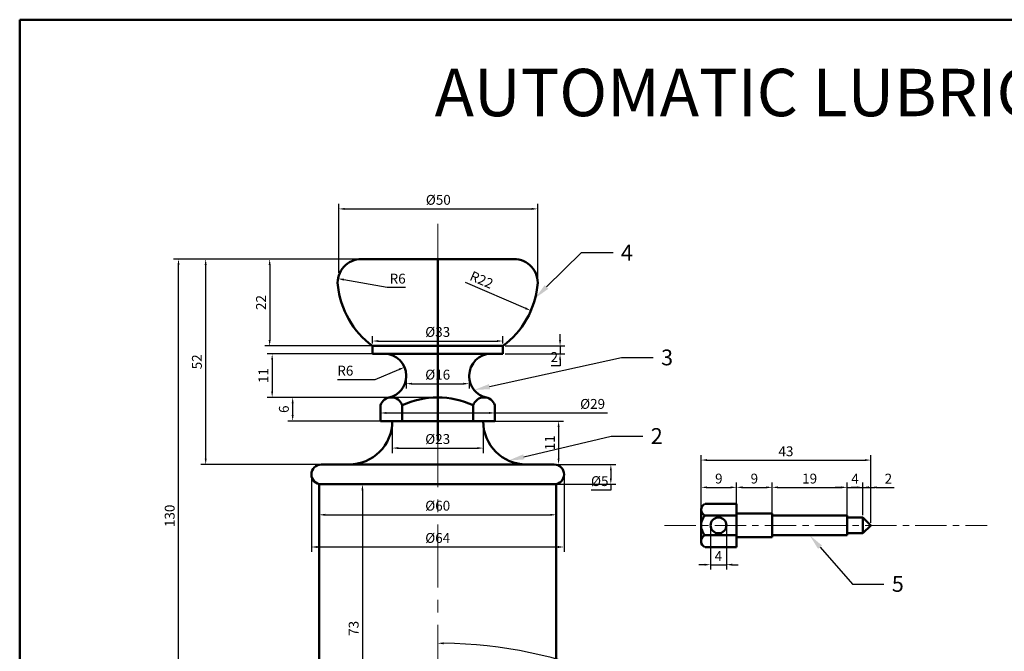
# Model space of a CAD drawing. Units: millimetres. Extents: x -414 to 17, y 81 to 417.
# Tile 6 of 7: x -414 to -165, y 257 to 417. Entities that reach past the tile are written whole.
import ezdxf
from ezdxf import colors
from ezdxf.entities.mleader import LeaderData, LeaderLine
from ezdxf.math import Vec2, Vec3

# ---------------------------------------------------------------- set-up
doc = ezdxf.new("R2010")
doc.units = ezdxf.units.MM
doc.header["$LTSCALE"] = 0.5
doc.linetypes.add('CENTER', pattern=[50.8, 31.75, -6.35, 6.35, -6.35])
for name, color, linetype, lineweight in [('M-CNTR', 1, 'CENTER', 18), ('M-DIMS', 2, 'Continuous', 25), ('M-OUTL', 7, 'Continuous', 50), ('M-TEXT', 3, 'Continuous', 25)]:
    doc.layers.add(name, color=color, linetype=linetype, lineweight=lineweight)
doc.styles.get("Standard").update_dxf_attribs({"font": 'arial.ttf'})
doc.dimstyles.new('ISO-25', dxfattribs={"dimtxt": 2.5, "dimasz": 1.5, "dimexe": 1.25, "dimexo": 0.625, "dimtad": 1, "dimtoh": 1, "dimdec": 0, "dimtxsty": 'Standard', "dimcen": 2.5, "dimadec": 0, "dimazin": 0, "dimtfac": 1, "dimtdec": 0, "dimtmove": 0, "dimatfit": 3, "dimfxl": 1, "dimarcsym": 0})

# ---------------------------------------------------------------- blocks, each defined once
blk = doc.blocks.new('*D1')
at = {"layer": 'Defpoints', "color": 0, "ltscale": 0.5, "transparency": 16777216}
for p in [(-283.16, 369.18), (-333.52, 352.37), (-283.16, 350.47)]:
    blk.add_point(p, dxfattribs=at)
at = {"layer": 'M-DIMS', "color": 0, "lineweight": -2, "ltscale": 0.5, "transparency": 16777216}
for p, q in [((-333.52, 353), (-333.52, 370.43)), ((-332.02, 369.18), (-284.66, 369.18)), ((-283.16, 351.09), (-283.16, 370.43))]:
    blk.add_line(p, q, dxfattribs=at)
at = {"layer": 'M-DIMS', "color": 0, "ltscale": 0.5, "transparency": 16777216}
for points in [[(-332.02, 369.43), (-332.02, 368.93), (-333.52, 369.18)], [(-284.66, 369.43), (-284.66, 368.93), (-283.16, 369.18)]]:
    blk.add_solid(points, dxfattribs=at)
at = {"layer": 'M-DIMS', "color": 0, "ltscale": 0.5, "transparency": 16777216, "insert": (-308.34, 371.15), "char_height": 2.5, "attachment_point": 5}
blk.add_mtext('%%C50', dxfattribs=at)
blk = doc.blocks.new('*D2')
at = {"layer": 'Defpoints', "color": 0, "ltscale": 0.5, "transparency": 16777216}
for p in [(-367.26, 356.47), (-319.11, 356.47), (-319.11, 304.46)]:
    blk.add_point(p, dxfattribs=at)
at = {"layer": 'M-DIMS', "color": 0, "lineweight": -2, "ltscale": 0.5, "transparency": 16777216}
for p, q in [((-319.74, 356.47), (-368.51, 356.47)), ((-367.26, 305.96), (-367.26, 354.97)), ((-319.74, 304.46), (-368.51, 304.46))]:
    blk.add_line(p, q, dxfattribs=at)
at = {"layer": 'M-DIMS', "color": 0, "ltscale": 0.5, "transparency": 16777216}
for points in [[(-367.51, 354.97), (-367.01, 354.97), (-367.26, 356.47)], [(-367.51, 305.96), (-367.01, 305.96), (-367.26, 304.46)]]:
    blk.add_solid(points, dxfattribs=at)
at = {"layer": 'M-DIMS', "color": 0, "ltscale": 0.5, "transparency": 16777216, "insert": (-369.16, 330.46), "char_height": 2.5, "attachment_point": 5, "rotation": 90}
blk.add_mtext('52', dxfattribs=at)
blk = doc.blocks.new('*D3')
at = {"layer": 'Defpoints', "color": 0, "ltscale": 0.5, "transparency": 16777216}
for p in [(-339.99, 356.47), (-351.05, 334.47), (-315.35, 334.47)]:
    blk.add_point(p, dxfattribs=at)
at = {"layer": 'M-DIMS', "color": 0, "lineweight": -2, "ltscale": 0.5, "transparency": 16777216}
for p, q in [((-340.61, 356.47), (-352.3, 356.47)), ((-351.05, 354.97), (-351.05, 335.97)), ((-315.97, 334.47), (-352.3, 334.47))]:
    blk.add_line(p, q, dxfattribs=at)
at = {"layer": 'M-DIMS', "color": 0, "ltscale": 0.5, "transparency": 16777216}
for points in [[(-351.3, 354.97), (-350.8, 354.97), (-351.05, 356.47)], [(-351.3, 335.97), (-350.8, 335.97), (-351.05, 334.47)]]:
    blk.add_solid(points, dxfattribs=at)
at = {"layer": 'M-DIMS', "color": 0, "ltscale": 0.5, "transparency": 16777216, "insert": (-352.93, 345.47), "char_height": 2.5, "attachment_point": 5, "rotation": 90}
blk.add_mtext('22', dxfattribs=at)
blk = doc.blocks.new('*D4')
at = {"layer": 'Defpoints', "color": 0, "ltscale": 0.5, "transparency": 16777216}
for p in [(-291.99, 334.47), (-291.99, 332.47), (-277.5, 332.47)]:
    blk.add_point(p, dxfattribs=at)
at = {"layer": 'M-DIMS', "color": 0, "lineweight": -2, "ltscale": 0.5, "transparency": 16777216}
for p, q in [((-277.5, 335.97), (-277.5, 337.47)), ((-291.37, 334.47), (-276.25, 334.47)), ((-277.5, 334.47), (-277.5, 332.47)), ((-291.37, 332.47), (-276.25, 332.47)), ((-277.5, 329.47), (-279.78, 329.47)), ((-277.5, 330.97), (-277.5, 329.47))]:
    blk.add_line(p, q, dxfattribs=at)
at = {"layer": 'M-DIMS', "color": 0, "ltscale": 0.5, "transparency": 16777216}
for points in [[(-277.75, 335.97), (-277.25, 335.97), (-277.5, 334.47)], [(-277.75, 330.97), (-277.25, 330.97), (-277.5, 332.47)]]:
    blk.add_solid(points, dxfattribs=at)
at = {"layer": 'M-DIMS', "color": 0, "ltscale": 0.5, "transparency": 16777216, "insert": (-278.95, 331.35), "char_height": 2.5, "attachment_point": 5}
blk.add_mtext('2', dxfattribs=at)
blk = doc.blocks.new('*D5')
at = {"layer": 'Defpoints', "color": 0, "ltscale": 0.5, "transparency": 16777216}
for p in [(-316.49, 326.78), (-300.49, 326.78), (-300.49, 324.92)]:
    blk.add_point(p, dxfattribs=at)
at = {"layer": 'M-DIMS', "color": 0, "lineweight": -2, "ltscale": 0.5, "transparency": 16777216}
for p, q in [((-316.49, 326.15), (-316.49, 323.67)), ((-314.99, 324.92), (-301.99, 324.92)), ((-300.49, 326.15), (-300.49, 323.67))]:
    blk.add_line(p, q, dxfattribs=at)
at = {"layer": 'M-DIMS', "color": 0, "ltscale": 0.5, "transparency": 16777216}
for points in [[(-314.99, 325.17), (-314.99, 324.67), (-316.49, 324.92)], [(-301.99, 325.17), (-301.99, 324.67), (-300.49, 324.92)]]:
    blk.add_solid(points, dxfattribs=at)
at = {"layer": 'M-DIMS', "color": 0, "ltscale": 0.5, "transparency": 16777216, "insert": (-308.49, 326.89), "char_height": 2.5, "attachment_point": 5}
blk.add_mtext('%%C16', dxfattribs=at)
blk = doc.blocks.new('*D6')
at = {"layer": 'Defpoints', "color": 0, "ltscale": 0.5, "transparency": 16777216}
for p in [(-308.49, 332.47), (-350.42, 321.46), (-308.49, 321.46)]:
    blk.add_point(p, dxfattribs=at)
at = {"layer": 'M-DIMS', "color": 0, "lineweight": -2, "ltscale": 0.5, "transparency": 16777216}
for p, q in [((-309.12, 332.47), (-351.67, 332.47)), ((-350.42, 330.97), (-350.42, 322.96)), ((-309.12, 321.46), (-351.67, 321.46))]:
    blk.add_line(p, q, dxfattribs=at)
at = {"layer": 'M-DIMS', "color": 0, "ltscale": 0.5, "transparency": 16777216}
for points in [[(-350.67, 330.97), (-350.17, 330.97), (-350.42, 332.47)], [(-350.67, 322.96), (-350.17, 322.96), (-350.42, 321.46)]]:
    blk.add_solid(points, dxfattribs=at)
at = {"layer": 'M-DIMS', "color": 0, "ltscale": 0.5, "transparency": 16777216, "insert": (-352.31, 326.96), "char_height": 2.5, "attachment_point": 5, "rotation": 90}
blk.add_mtext('11', dxfattribs=at)
blk = doc.blocks.new('*D7')
at = {"layer": 'Defpoints', "color": 0, "ltscale": 0.5, "transparency": 16777216}
for p in [(-308.49, 321.46), (-345.23, 315.46), (-308.49, 315.46)]:
    blk.add_point(p, dxfattribs=at)
at = {"layer": 'M-DIMS', "color": 0, "lineweight": -2, "ltscale": 0.5, "transparency": 16777216}
for p, q in [((-309.12, 321.46), (-346.48, 321.46)), ((-345.23, 319.96), (-345.23, 316.96)), ((-309.12, 315.46), (-346.48, 315.46))]:
    blk.add_line(p, q, dxfattribs=at)
at = {"layer": 'M-DIMS', "color": 0, "ltscale": 0.5, "transparency": 16777216}
for points in [[(-345.48, 319.96), (-344.98, 319.96), (-345.23, 321.46)], [(-345.48, 316.96), (-344.98, 316.96), (-345.23, 315.46)]]:
    blk.add_solid(points, dxfattribs=at)
at = {"layer": 'M-DIMS', "color": 0, "ltscale": 0.5, "transparency": 16777216, "insert": (-347.13, 318.46), "char_height": 2.5, "attachment_point": 5, "rotation": 90}
blk.add_mtext('6', dxfattribs=at)
blk = doc.blocks.new('*D8')
at = {"layer": 'Defpoints', "color": 0, "ltscale": 0.5, "transparency": 16777216}
for p in [(-308.49, 315.46), (-308.49, 304.46), (-277.87, 304.46)]:
    blk.add_point(p, dxfattribs=at)
at = {"layer": 'M-DIMS', "color": 0, "lineweight": -2, "ltscale": 0.5, "transparency": 16777216}
for p, q in [((-307.87, 315.46), (-276.62, 315.46)), ((-277.87, 313.96), (-277.87, 305.96)), ((-307.87, 304.46), (-276.62, 304.46))]:
    blk.add_line(p, q, dxfattribs=at)
at = {"layer": 'M-DIMS', "color": 0, "ltscale": 0.5, "transparency": 16777216}
for points in [[(-278.12, 313.96), (-277.62, 313.96), (-277.87, 315.46)], [(-278.12, 305.96), (-277.62, 305.96), (-277.87, 304.46)]]:
    blk.add_solid(points, dxfattribs=at)
at = {"layer": 'M-DIMS', "color": 0, "ltscale": 0.5, "transparency": 16777216, "insert": (-279.75, 309.96), "char_height": 2.5, "attachment_point": 5, "rotation": 90}
blk.add_mtext('11', dxfattribs=at)
blk = doc.blocks.new('*D9')
at = {"layer": 'Defpoints', "color": 0, "ltscale": 0.5, "transparency": 16777216}
for p in [(-324.99, 334.47), (-291.99, 335.72), (-291.99, 334.47)]:
    blk.add_point(p, dxfattribs=at)
at = {"layer": 'M-DIMS', "color": 0, "lineweight": -2, "ltscale": 0.5, "transparency": 16777216}
for p, q in [((-324.99, 335.09), (-324.99, 336.97)), ((-291.99, 335.09), (-291.99, 336.97)), ((-323.49, 335.72), (-293.49, 335.72))]:
    blk.add_line(p, q, dxfattribs=at)
at = {"layer": 'M-DIMS', "color": 0, "ltscale": 0.5, "transparency": 16777216}
for points in [[(-323.49, 335.97), (-323.49, 335.47), (-324.99, 335.72)], [(-293.49, 335.97), (-293.49, 335.47), (-291.99, 335.72)]]:
    blk.add_solid(points, dxfattribs=at)
at = {"layer": 'M-DIMS', "color": 0, "ltscale": 0.5, "transparency": 16777216, "insert": (-308.49, 337.7), "char_height": 2.5, "attachment_point": 5}
blk.add_mtext('%%C33', dxfattribs=at)
blk = doc.blocks.new('*D10')
at = {"layer": 'Defpoints', "color": 0, "ltscale": 0.5, "transparency": 16777216}
for p in [(-333.74, 351.52), (-327.83, 350.47)]:
    blk.add_point(p, dxfattribs=at)
at = {"layer": 'M-DIMS', "color": 0, "lineweight": -2, "ltscale": 0.5, "transparency": 16777216}
for p, q in [((-321.28, 349.3), (-332.26, 351.26)), ((-316.62, 349.3), (-321.28, 349.3))]:
    blk.add_line(p, q, dxfattribs=at)
at = {"layer": 'M-DIMS', "color": 0, "ltscale": 0.5, "transparency": 16777216}
blk.add_solid([(-332.22, 351.5), (-332.3, 351.01), (-333.74, 351.52)], dxfattribs=at)
at = {"layer": 'M-DIMS', "color": 0, "ltscale": 0.5, "transparency": 16777216, "insert": (-318.64, 351.2), "char_height": 2.5, "attachment_point": 5}
blk.add_mtext('R6', dxfattribs=at)
blk = doc.blocks.new('*D11')
at = {"layer": 'Defpoints', "color": 0, "ltscale": 0.5, "transparency": 16777216}
for p in [(-305.07, 352.16), (-284.88, 343.42)]:
    blk.add_point(p, dxfattribs=at)
at = {"layer": 'M-DIMS', "color": 0, "lineweight": -2, "ltscale": 0.5, "transparency": 16777216}
blk.add_line((-301.55, 350.64), (-286.26, 344.01), dxfattribs=at)
at = {"layer": 'M-DIMS', "color": 0, "ltscale": 0.5, "transparency": 16777216}
blk.add_solid([(-286.16, 344.24), (-286.36, 343.78), (-284.88, 343.42)], dxfattribs=at)
at = {"layer": 'M-DIMS', "color": 0, "ltscale": 0.5, "transparency": 16777216, "insert": (-297.5, 350.93), "char_height": 2.5, "attachment_point": 5, "rotation": 336.5806}
blk.add_mtext('R22', dxfattribs=at)
blk = doc.blocks.new('*D12')
at = {"layer": 'Defpoints', "color": 0, "ltscale": 0.5, "transparency": 16777216}
for p in [(-321.99, 326.97), (-316.92, 329.09)]:
    blk.add_point(p, dxfattribs=at)
at = {"layer": 'M-DIMS', "color": 0, "lineweight": -2, "ltscale": 0.5, "transparency": 16777216}
for p, q in [((-324.3, 326), (-318.3, 328.51)), ((-333.9, 326), (-324.3, 326))]:
    blk.add_line(p, q, dxfattribs=at)
at = {"layer": 'M-DIMS', "color": 0, "ltscale": 0.5, "transparency": 16777216}
blk.add_solid([(-318.4, 328.74), (-318.21, 328.28), (-316.92, 329.09)], dxfattribs=at)
at = {"layer": 'M-DIMS', "color": 0, "ltscale": 0.5, "transparency": 16777216, "insert": (-331.89, 327.9), "char_height": 2.5, "attachment_point": 5}
blk.add_mtext('R6', dxfattribs=at)
blk = doc.blocks.new('*D13')
at = {"layer": 'Defpoints', "color": 0, "ltscale": 0.5, "transparency": 16777216}
for p in [(-293.99, 317.51), (-322.99, 315.46), (-293.99, 315.46)]:
    blk.add_point(p, dxfattribs=at)
at = {"layer": 'M-DIMS', "color": 0, "lineweight": -2, "ltscale": 0.5, "transparency": 16777216}
for p, q in [((-322.99, 316.09), (-322.99, 318.76)), ((-321.49, 317.51), (-295.49, 317.51)), ((-293.99, 316.09), (-293.99, 318.76)), ((-293.99, 317.51), (-265.48, 317.51))]:
    blk.add_line(p, q, dxfattribs=at)
at = {"layer": 'M-DIMS', "color": 0, "ltscale": 0.5, "transparency": 16777216}
for points in [[(-321.49, 317.76), (-321.49, 317.26), (-322.99, 317.51)], [(-295.49, 317.76), (-295.49, 317.26), (-293.99, 317.51)]]:
    blk.add_solid(points, dxfattribs=at)
at = {"layer": 'M-DIMS', "color": 0, "ltscale": 0.5, "transparency": 16777216, "insert": (-269.26, 319.48), "char_height": 2.5, "attachment_point": 5}
blk.add_mtext('%%C29', dxfattribs=at)
blk = doc.blocks.new('*D14')
at = {"layer": 'Defpoints', "color": 0, "ltscale": 0.5, "transparency": 16777216}
for p in [(-319.99, 315.46), (-296.99, 315.46), (-296.99, 308.62)]:
    blk.add_point(p, dxfattribs=at)
at = {"layer": 'M-DIMS', "color": 0, "lineweight": -2, "ltscale": 0.5, "transparency": 16777216}
for p, q in [((-319.99, 314.84), (-319.99, 307.37)), ((-296.99, 314.84), (-296.99, 307.37)), ((-318.49, 308.62), (-298.49, 308.62))]:
    blk.add_line(p, q, dxfattribs=at)
at = {"layer": 'M-DIMS', "color": 0, "ltscale": 0.5, "transparency": 16777216}
for points in [[(-318.49, 308.87), (-318.49, 308.37), (-319.99, 308.62)], [(-298.49, 308.87), (-298.49, 308.37), (-296.99, 308.62)]]:
    blk.add_solid(points, dxfattribs=at)
at = {"layer": 'M-DIMS', "color": 0, "ltscale": 0.5, "transparency": 16777216, "insert": (-308.49, 310.59), "char_height": 2.5, "attachment_point": 5}
blk.add_mtext('%%C23', dxfattribs=at)
blk = doc.blocks.new('*D15')
at = {"layer": 'Defpoints', "color": 0, "ltscale": 0.5, "transparency": 16777216}
for p in [(-282.49, 304.46), (-282.49, 299.46), (-264.64, 299.46)]:
    blk.add_point(p, dxfattribs=at)
at = {"layer": 'M-DIMS', "color": 0, "lineweight": -2, "ltscale": 0.5, "transparency": 16777216}
for p, q in [((-281.87, 304.46), (-263.39, 304.46)), ((-264.64, 302.96), (-264.64, 300.96)), ((-281.87, 299.46), (-263.39, 299.46)), ((-264.64, 299.46), (-264.64, 297.96)), ((-264.64, 297.96), (-269.64, 297.96))]:
    blk.add_line(p, q, dxfattribs=at)
at = {"layer": 'M-DIMS', "color": 0, "ltscale": 0.5, "transparency": 16777216}
for points in [[(-264.89, 302.96), (-264.39, 302.96), (-264.64, 304.46)], [(-264.89, 300.96), (-264.39, 300.96), (-264.64, 299.46)]]:
    blk.add_solid(points, dxfattribs=at)
at = {"layer": 'M-DIMS', "color": 0, "ltscale": 0.5, "transparency": 16777216, "insert": (-267.45, 299.93), "char_height": 2.5, "attachment_point": 5}
blk.add_mtext('%%C5', dxfattribs=at)
blk = doc.blocks.new('*D16')
at = {"layer": 'Defpoints', "color": 0, "ltscale": 0.5, "transparency": 16777216}
for p in [(-340.49, 301.96), (-276.49, 301.96), (-276.49, 283.57)]:
    blk.add_point(p, dxfattribs=at)
at = {"layer": 'M-DIMS', "color": 0, "lineweight": -2, "ltscale": 0.5, "transparency": 16777216}
for p, q in [((-340.49, 301.34), (-340.49, 282.32)), ((-276.49, 301.34), (-276.49, 282.32)), ((-338.99, 283.57), (-277.99, 283.57))]:
    blk.add_line(p, q, dxfattribs=at)
at = {"layer": 'M-DIMS', "color": 0, "ltscale": 0.5, "transparency": 16777216}
for points in [[(-338.99, 283.82), (-338.99, 283.32), (-340.49, 283.57)], [(-277.99, 283.82), (-277.99, 283.32), (-276.49, 283.57)]]:
    blk.add_solid(points, dxfattribs=at)
at = {"layer": 'M-DIMS', "color": 0, "ltscale": 0.5, "transparency": 16777216, "insert": (-308.49, 285.54), "char_height": 2.5, "attachment_point": 5}
blk.add_mtext('%%C64', dxfattribs=at)
blk = doc.blocks.new('*D17')
at = {"layer": 'Defpoints', "color": 0, "ltscale": 0.5, "transparency": 16777216}
for p in [(-338.49, 294.85), (-278.49, 294.85), (-278.49, 291.72)]:
    blk.add_point(p, dxfattribs=at)
at = {"layer": 'M-DIMS', "color": 0, "lineweight": -2, "ltscale": 0.5, "transparency": 16777216}
for p, q in [((-338.49, 294.23), (-338.49, 290.47)), ((-278.49, 294.23), (-278.49, 290.47)), ((-336.99, 291.72), (-279.99, 291.72))]:
    blk.add_line(p, q, dxfattribs=at)
at = {"layer": 'M-DIMS', "color": 0, "ltscale": 0.5, "transparency": 16777216}
for points in [[(-336.99, 291.97), (-336.99, 291.47), (-338.49, 291.72)], [(-279.99, 291.97), (-279.99, 291.47), (-278.49, 291.72)]]:
    blk.add_solid(points, dxfattribs=at)
at = {"layer": 'M-DIMS', "color": 0, "ltscale": 0.5, "transparency": 16777216, "insert": (-308.49, 293.7), "char_height": 2.5, "attachment_point": 5}
blk.add_mtext('%%C60', dxfattribs=at)
blk = doc.blocks.new('*D18')
at = {"layer": 'Defpoints', "color": 0, "ltscale": 0.5, "transparency": 16777216}
for p in [(-328.26, 299.46), (-328.26, 226.46), (-327.55, 226.46)]:
    blk.add_point(p, dxfattribs=at)
at = {"layer": 'M-DIMS', "color": 0, "lineweight": -2, "ltscale": 0.5, "transparency": 16777216}
for p, q in [((-327.63, 299.46), (-326.3, 299.46)), ((-327.55, 297.96), (-327.55, 227.96)), ((-327.63, 226.46), (-326.3, 226.46))]:
    blk.add_line(p, q, dxfattribs=at)
at = {"layer": 'M-DIMS', "color": 0, "ltscale": 0.5, "transparency": 16777216}
for points in [[(-327.8, 297.96), (-327.3, 297.96), (-327.55, 299.46)], [(-327.8, 227.96), (-327.3, 227.96), (-327.55, 226.46)]]:
    blk.add_solid(points, dxfattribs=at)
at = {"layer": 'M-DIMS', "color": 0, "ltscale": 0.5, "transparency": 16777216, "insert": (-329.45, 262.96), "char_height": 2.5, "attachment_point": 5, "rotation": 90}
blk.add_mtext('73', dxfattribs=at)
blk = doc.blocks.new('*D39')
at = {"layer": 'Defpoints', "color": 0, "ltscale": 0.5, "transparency": 16777216}
for p in [(-374.14, 356.47), (-308.49, 356.47), (-361.11, 226.46)]:
    blk.add_point(p, dxfattribs=at)
at = {"layer": 'M-DIMS', "color": 0, "lineweight": -2, "ltscale": 0.5, "transparency": 16777216}
for p, q in [((-309.12, 356.47), (-375.39, 356.47)), ((-374.14, 227.96), (-374.14, 354.97)), ((-361.74, 226.46), (-375.39, 226.46))]:
    blk.add_line(p, q, dxfattribs=at)
at = {"layer": 'M-DIMS', "color": 0, "ltscale": 0.5, "transparency": 16777216}
for points in [[(-374.39, 354.97), (-373.89, 354.97), (-374.14, 356.47)], [(-374.39, 227.96), (-373.89, 227.96), (-374.14, 226.46)]]:
    blk.add_solid(points, dxfattribs=at)
at = {"layer": 'M-DIMS', "color": 0, "ltscale": 0.5, "transparency": 16777216, "insert": (-376.05, 291.46), "char_height": 2.5, "attachment_point": 5, "rotation": 90}
blk.add_mtext('130', dxfattribs=at)
blk = doc.blocks.new('*D71')
at = {"layer": 'Defpoints', "color": 0, "ltscale": 0.5, "transparency": 16777216}
for p in [(-198.79, 305.58), (-241.79, 289.04), (-198.79, 289.04)]:
    blk.add_point(p, dxfattribs=at)
at = {"layer": 'M-DIMS', "color": 0, "lineweight": -2, "ltscale": 0.5, "transparency": 16777216}
for p, q in [((-241.79, 289.67), (-241.79, 306.83)), ((-198.79, 289.67), (-198.79, 306.83)), ((-240.29, 305.58), (-200.29, 305.58))]:
    blk.add_line(p, q, dxfattribs=at)
at = {"layer": 'M-DIMS', "color": 0, "ltscale": 0.5, "transparency": 16777216}
for points in [[(-240.29, 305.83), (-240.29, 305.33), (-241.79, 305.58)], [(-200.29, 305.83), (-200.29, 305.33), (-198.79, 305.58)]]:
    blk.add_solid(points, dxfattribs=at)
at = {"layer": 'M-DIMS', "color": 0, "ltscale": 0.5, "transparency": 16777216, "insert": (-220.29, 307.48), "char_height": 2.5, "attachment_point": 5}
blk.add_mtext('43', dxfattribs=at)
blk = doc.blocks.new('*D72')
at = {"layer": 'Defpoints', "color": 0, "ltscale": 0.5, "transparency": 16777216}
for p in [(-232.79, 298.67), (-241.79, 289.04), (-232.79, 289.04)]:
    blk.add_point(p, dxfattribs=at)
at = {"layer": 'M-DIMS', "color": 0, "lineweight": -2, "ltscale": 0.5, "transparency": 16777216}
for p, q in [((-241.79, 289.67), (-241.79, 299.92)), ((-232.79, 289.67), (-232.79, 299.92)), ((-240.29, 298.67), (-234.29, 298.67))]:
    blk.add_line(p, q, dxfattribs=at)
at = {"layer": 'M-DIMS', "color": 0, "ltscale": 0.5, "transparency": 16777216}
for points in [[(-240.29, 298.92), (-240.29, 298.42), (-241.79, 298.67)], [(-234.29, 298.92), (-234.29, 298.42), (-232.79, 298.67)]]:
    blk.add_solid(points, dxfattribs=at)
at = {"layer": 'M-DIMS', "color": 0, "ltscale": 0.5, "transparency": 16777216, "insert": (-237.29, 300.57), "char_height": 2.5, "attachment_point": 5}
blk.add_mtext('9', dxfattribs=at)
blk = doc.blocks.new('*D73')
at = {"layer": 'Defpoints', "color": 0, "ltscale": 0.5, "transparency": 16777216}
for p in [(-223.79, 298.67), (-232.79, 289.04), (-223.79, 289.04)]:
    blk.add_point(p, dxfattribs=at)
at = {"layer": 'M-DIMS', "color": 0, "lineweight": -2, "ltscale": 0.5, "transparency": 16777216}
for p, q in [((-232.79, 289.67), (-232.79, 299.92)), ((-223.79, 289.67), (-223.79, 299.92)), ((-231.29, 298.67), (-225.29, 298.67))]:
    blk.add_line(p, q, dxfattribs=at)
at = {"layer": 'M-DIMS', "color": 0, "ltscale": 0.5, "transparency": 16777216}
for points in [[(-231.29, 298.92), (-231.29, 298.42), (-232.79, 298.67)], [(-225.29, 298.92), (-225.29, 298.42), (-223.79, 298.67)]]:
    blk.add_solid(points, dxfattribs=at)
at = {"layer": 'M-DIMS', "color": 0, "ltscale": 0.5, "transparency": 16777216, "insert": (-228.29, 300.57), "char_height": 2.5, "attachment_point": 5}
blk.add_mtext('9', dxfattribs=at)
blk = doc.blocks.new('*D74')
at = {"layer": 'Defpoints', "color": 0, "ltscale": 0.5, "transparency": 16777216}
for p in [(-204.79, 298.67), (-223.79, 289.04), (-204.79, 289.04)]:
    blk.add_point(p, dxfattribs=at)
at = {"layer": 'M-DIMS', "color": 0, "lineweight": -2, "ltscale": 0.5, "transparency": 16777216}
for p, q in [((-223.79, 289.67), (-223.79, 299.92)), ((-204.79, 289.67), (-204.79, 299.92)), ((-222.29, 298.67), (-206.29, 298.67))]:
    blk.add_line(p, q, dxfattribs=at)
at = {"layer": 'M-DIMS', "color": 0, "ltscale": 0.5, "transparency": 16777216}
for points in [[(-222.29, 298.92), (-222.29, 298.42), (-223.79, 298.67)], [(-206.29, 298.92), (-206.29, 298.42), (-204.79, 298.67)]]:
    blk.add_solid(points, dxfattribs=at)
at = {"layer": 'M-DIMS', "color": 0, "ltscale": 0.5, "transparency": 16777216, "insert": (-214.29, 300.57), "char_height": 2.5, "attachment_point": 5}
blk.add_mtext('19', dxfattribs=at)
blk = doc.blocks.new('*D75')
at = {"layer": 'Defpoints', "color": 0, "ltscale": 0.5, "transparency": 16777216}
for p in [(-200.79, 298.67), (-204.79, 291.04), (-200.79, 291.04)]:
    blk.add_point(p, dxfattribs=at)
at = {"layer": 'M-DIMS', "color": 0, "lineweight": -2, "ltscale": 0.5, "transparency": 16777216}
for p, q in [((-204.79, 291.67), (-204.79, 299.92)), ((-200.79, 291.67), (-200.79, 299.92)), ((-206.29, 298.67), (-207.79, 298.67)), ((-204.79, 298.67), (-200.79, 298.67)), ((-199.29, 298.67), (-197.79, 298.67))]:
    blk.add_line(p, q, dxfattribs=at)
at = {"layer": 'M-DIMS', "color": 0, "ltscale": 0.5, "transparency": 16777216}
for points in [[(-206.29, 298.92), (-206.29, 298.42), (-204.79, 298.67)], [(-199.29, 298.92), (-199.29, 298.42), (-200.79, 298.67)]]:
    blk.add_solid(points, dxfattribs=at)
at = {"layer": 'M-DIMS', "color": 0, "ltscale": 0.5, "transparency": 16777216, "insert": (-202.79, 300.54), "char_height": 2.5, "attachment_point": 5}
blk.add_mtext('4', dxfattribs=at)
blk = doc.blocks.new('*D76')
at = {"layer": 'Defpoints', "color": 0, "ltscale": 0.5, "transparency": 16777216}
for p in [(-198.79, 298.67), (-200.79, 291.04), (-198.79, 290.27)]:
    blk.add_point(p, dxfattribs=at)
at = {"layer": 'M-DIMS', "color": 0, "lineweight": -2, "ltscale": 0.5, "transparency": 16777216}
for p, q in [((-200.79, 291.67), (-200.79, 299.92)), ((-198.79, 290.9), (-198.79, 299.92)), ((-202.29, 298.67), (-203.79, 298.67)), ((-200.79, 298.67), (-198.79, 298.67)), ((-197.29, 298.67), (-192.89, 298.67))]:
    blk.add_line(p, q, dxfattribs=at)
at = {"layer": 'M-DIMS', "color": 0, "ltscale": 0.5, "transparency": 16777216}
for points in [[(-202.29, 298.92), (-202.29, 298.42), (-200.79, 298.67)], [(-197.29, 298.92), (-197.29, 298.42), (-198.79, 298.67)]]:
    blk.add_solid(points, dxfattribs=at)
at = {"layer": 'M-DIMS', "color": 0, "ltscale": 0.5, "transparency": 16777216, "insert": (-194.34, 300.55), "char_height": 2.5, "attachment_point": 5}
blk.add_mtext('2', dxfattribs=at)
blk = doc.blocks.new('*D77')
at = {"layer": 'Defpoints', "color": 0, "ltscale": 0.5, "transparency": 16777216}
for p in [(-239.38, 289.04), (-235.38, 289.04), (-235.38, 279.09)]:
    blk.add_point(p, dxfattribs=at)
at = {"layer": 'M-DIMS', "color": 0, "lineweight": -2, "ltscale": 0.5, "transparency": 16777216}
for p, q in [((-239.38, 288.42), (-239.38, 277.84)), ((-235.38, 288.42), (-235.38, 277.84)), ((-240.88, 279.09), (-242.38, 279.09)), ((-239.38, 279.09), (-235.38, 279.09)), ((-233.88, 279.09), (-232.38, 279.09))]:
    blk.add_line(p, q, dxfattribs=at)
at = {"layer": 'M-DIMS', "color": 0, "ltscale": 0.5, "transparency": 16777216}
for points in [[(-240.88, 279.34), (-240.88, 278.84), (-239.38, 279.09)], [(-233.88, 279.34), (-233.88, 278.84), (-235.38, 279.09)]]:
    blk.add_solid(points, dxfattribs=at)
at = {"layer": 'M-DIMS', "color": 0, "ltscale": 0.5, "transparency": 16777216, "insert": (-237.38, 280.97), "char_height": 2.5, "attachment_point": 5}
blk.add_mtext('4', dxfattribs=at)
blk = doc.blocks.new('*D78')
at = {"layer": 'Defpoints', "color": 0, "ltscale": 0.5, "transparency": 16777216}
for p in [(-308.49, 365.43), (-250.63, 243.68), (-212.22, 239.73), (-308.49, 230.96), (-308.49, 143.46)]:
    blk.add_point(p, dxfattribs=at)
at = {"layer": 'M-DIMS', "color": 0, "lineweight": -2, "ltscale": 0.5, "transparency": 16777216}
blk.add_arc((-308.49, 143.46), 115.73, 45.7426, 89.2574, dxfattribs=at)
at = {"layer": 'M-DIMS', "color": 0, "ltscale": 0.5, "transparency": 16777216}
for points in [[(-306.99, 258.93), (-306.99, 259.43), (-308.49, 259.19)], [(-227.55, 226.52), (-227.9, 226.17), (-226.66, 225.29)]]:
    blk.add_solid(points, dxfattribs=at)
at = {"layer": 'M-DIMS', "color": 0, "ltscale": 0.5, "transparency": 16777216, "insert": (-263.48, 252.13), "char_height": 2.5, "attachment_point": 5, "rotation": 337.5}
blk.add_mtext('45°', dxfattribs=at)

msp = doc.modelspace()

# ---------------------------------------------------------------- linework, layer by layer
at = {"layer": 'M-CNTR'}
msp.add_line((-308.49, 365.43), (-308.49, 230.96), dxfattribs=at)
at = {"layer": 'M-CNTR', "ltscale": 0.5}
msp.add_line((-251.03, 289.04), (-169.29, 289.04), dxfattribs=at)
at = {"layer": 'M-OUTL', "ltscale": 0.5}
for p, q in [((-327.83, 356.47), (-289.16, 356.47)), ((-308.49, 356.47), (-308.49, 334.47)), ((-324.99, 334.47), (-291.99, 334.47)), ((-324.99, 332.47), (-324.99, 334.47)), ((-291.99, 332.47), (-291.99, 334.47)), ((-324.99, 332.47), (-291.99, 332.47)), ((-240.79, 294.54), (-232.79, 294.54)), ((-232.79, 283.54), (-232.79, 294.54)), ((-241.79, 285.04), (-241.79, 293.04)), ((-232.79, 286.04), (-232.79, 292.04)), ((-232.79, 292.04), (-223.79, 292.04)), ((-223.79, 292.04), (-223.79, 286.04)), ((-240.79, 291.54), (-232.79, 291.54)), ((-223.79, 291.54), (-204.79, 291.54)), ((-223.79, 286.54), (-223.79, 291.54)), ((-204.79, 291.54), (-204.79, 286.54)), ((-204.79, 291.04), (-200.79, 291.04)), ((-204.79, 287.04), (-204.79, 291.04)), ((-200.79, 291.04), (-200.79, 287.04)), ((-198.79, 289.04), (-200.79, 291.04)), ((-200.79, 287.04), (-204.79, 287.04)), ((-200.79, 287.04), (-198.79, 289.04)), ((-240.79, 286.54), (-232.79, 286.54)), ((-232.79, 286.04), (-223.79, 286.04)), ((-204.79, 286.54), (-223.79, 286.54)), ((-240.79, 283.54), (-232.79, 283.54))]:
    msp.add_line(p, q, dxfattribs=at)
at = {"layer": 'M-OUTL'}
for p, q in [((-308.49, 310.61), (-308.49, 339.44)), ((-291.99, 332.47), (-308.49, 332.47)), ((-316.49, 326.78), (-316.49, 326.97)), ((-300.49, 326.78), (-300.49, 326.97)), ((-322.99, 319.46), (-322.99, 315.46)), ((-317.49, 319.46), (-317.49, 315.46)), ((-299.49, 319.46), (-299.49, 315.46)), ((-293.99, 315.46), (-293.99, 319.46)), ((-322.99, 315.46), (-293.99, 315.46)), ((-319.99, 315.46), (-296.99, 315.46)), ((-308.49, 315.46), (-308.49, 310.61)), ((-337.99, 304.46), (-285.99, 304.46)), ((-285.99, 304.46), (-278.99, 304.46)), ((-340.49, 301.96), (-340.49, 301.96)), ((-276.49, 301.96), (-276.49, 301.96)), ((-338.49, 299.46), (-338.49, 226.46)), ((-337.99, 299.46), (-278.99, 299.46)), ((-278.49, 299.46), (-278.49, 226.46))]:
    msp.add_line(p, q, dxfattribs=at)
at = {"layer": 'M-OUTL', "ltscale": 0.5}
msp.add_lwpolyline([(-414.36, 417.09), (16.87, 417.09), (16.87, 80.66), (-414.36, 80.66)], close=True, dxfattribs=at)
msp.add_circle((-237.38, 289.04), 2, dxfattribs=at)
for centre, radius, start, end in [((-327.83, 350.47), 6, 90, 186.0758), ((-289.16, 350.47), 6, 353.9242, 90), ((-311.92, 352.16), 22, 186.0758, 233.5379), ((-305.07, 352.16), 22, 306.4621, 353.9242), ((-240.17, 293.04), 1.62, 112.6199, 247.3801), ((-238.17, 289.04), 3.62, 136.3972, 223.6028), ((-240.17, 285.04), 1.63, 112.6199, 247.3801)]:
    msp.add_arc(centre, radius, start, end, dxfattribs=at)
at = {"layer": 'M-OUTL'}
for centre, radius, start, end in [((-321.99, 326.97), 5.5, 0, 90), ((-294.99, 326.97), 5.5, 90, 180), ((-321.99, 326.78), 5.5, 282.0389, 0), ((-294.99, 326.78), 5.5, 180, 257.9615), ((-320.24, 318.57), 2.89, 17.923, 162.077), ((-308.49, 300.21), 21.25, 64.9424, 115.0576), ((-296.74, 318.57), 2.89, 17.9401, 162.0599), ((-330.99, 315.46), 11, 270, 0), ((-285.99, 315.46), 11, 180, 270), ((-337.99, 301.96), 2.5, 90, 180), ((-278.99, 301.96), 2.5, 0, 90), ((-337.99, 301.96), 2.5, 180, 270), ((-278.99, 301.96), 2.5, 270, 0)]:
    msp.add_arc(centre, radius, start, end, dxfattribs=at)

# ---------------------------------------------------------------- texts
at = {"layer": 'M-TEXT', "ltscale": 0.5, "insert": (-337.22, 404.65), "char_height": 12, "attachment_point": 1}
msp.add_mtext_dynamic_manual_height_columns('\\pxqc;AUTOMATIC LUBRICATOR', width=250.9828, gutter_width=12.5, heights=[0], dxfattribs=at)

# ---------------------------------------------------------------- dimensions: what is measured, and where the dimension line sits
at = {"layer": 'M-DIMS', "ltscale": 0.5}
for base, p1, p2, picture, middle in [((-283.16, 369.18), (-333.52, 352.37), (-283.16, 350.47), '*D1', (-308.34, 371.15)), ((-291.99, 335.72), (-324.99, 334.47), (-291.99, 334.47), '*D9', (-308.49, 337.7)), ((-300.49, 324.92), (-316.49, 326.78), (-300.49, 326.78), '*D5', (-308.49, 326.89)), ((-296.99, 308.62), (-319.99, 315.46), (-296.99, 315.46), '*D14', (-308.49, 310.59)), ((-276.49, 283.57), (-340.49, 301.96), (-276.49, 301.96), '*D16', (-308.49, 285.54)), ((-278.49, 291.72), (-338.49, 294.85), (-278.49, 294.85), '*D17', (-308.49, 293.7))]:
    dim = msp.add_linear_dim(base=base, p1=p1, p2=p2, text='%%C<>', dimstyle='ISO-25', override={"dimclrd": 0, "dimclre": 0, "dimclrt": 0}, dxfattribs=at)
    dim.commit()
    dim.dimension.update_dxf_attribs({"geometry": picture, "text_midpoint": middle})
dim = msp.add_angular_dim_2l(base=(-250.63, 243.68), line1=((-308.49, 365.43), (-308.49, 230.96)), line2=((-212.22, 239.73), (-308.49, 143.46)), dimstyle='ISO-25', override={"dimclrd": 0, "dimclre": 0, "dimclrt": 0}, dxfattribs=at)
dim.commit()
dim.dimension.update_dxf_attribs({"geometry": '*D78', "text_midpoint": (-263.48, 252.13)})
for base, p1, p2, picture, middle in [((-374.14, 356.47), (-361.11, 226.46), (-308.49, 356.47), '*D39', (-376.05, 291.46)), ((-367.26, 356.47), (-319.11, 304.46), (-319.11, 356.47), '*D2', (-369.16, 330.46)), ((-351.05, 334.47), (-339.99, 356.47), (-315.35, 334.47), '*D3', (-352.93, 345.47)), ((-277.5, 332.47), (-291.99, 334.47), (-291.99, 332.47), '*D4', (-278.95, 331.35)), ((-350.42, 321.46), (-308.49, 332.47), (-308.49, 321.46), '*D6', (-352.31, 326.96)), ((-345.23, 315.46), (-308.49, 321.46), (-308.49, 315.46), '*D7', (-347.13, 318.46)), ((-277.87, 304.46), (-308.49, 315.46), (-308.49, 304.46), '*D8', (-279.75, 309.96)), ((-327.55, 226.46), (-328.26, 299.46), (-328.26, 226.46), '*D18', (-329.45, 262.96))]:
    dim = msp.add_linear_dim(base=base, p1=p1, p2=p2, angle=90, dimstyle='ISO-25', override={"dimclrd": 0, "dimclre": 0, "dimclrt": 0}, dxfattribs=at)
    dim.commit()
    dim.dimension.update_dxf_attribs({"geometry": picture, "text_midpoint": middle})
for center, mpoint, picture, middle in [((-327.83, 350.47), (-333.74, 351.52), '*D10', (-321.28, 349.3)), ((-305.07, 352.16), (-284.88, 343.42), '*D11', (-298.25, 349.21)), ((-321.99, 326.97), (-316.92, 329.09), '*D12', (-331.89, 326))]:
    dim = msp.add_radius_dim(center=center, mpoint=mpoint, dimstyle='ISO-25', override={"dimclrd": 0, "dimclre": 0, "dimclrt": 0}, dxfattribs=at)
    dim.commit()
    dim.dimension.update_dxf_attribs({"geometry": picture, "text_midpoint": middle, "dimtype": 164})
dim = msp.add_linear_dim(base=(-293.99, 317.51), p1=(-322.99, 315.46), p2=(-293.99, 315.46), text='%%C<>', dimstyle='ISO-25', override={"dimclrd": 0, "dimclre": 0, "dimclrt": 0}, dxfattribs=at)
dim.commit()
dim.dimension.update_dxf_attribs({"geometry": '*D13', "text_midpoint": (-269.26, 317.51), "dimtype": 160})
for base, p1, p2, override, picture, middle in [((-198.79, 305.58), (-241.79, 289.04), (-198.79, 289.04), {"dimclrd": 0, "dimclre": 0, "dimclrt": 0}, '*D71', (-220.29, 307.48)), ((-232.79, 298.67), (-241.79, 289.04), (-232.79, 289.04), {"dimclrd": 0, "dimclre": 0, "dimclrt": 0, "dimtmove": 0}, '*D72', (-237.29, 300.57)), ((-198.79, 298.67), (-200.79, 291.04), (-198.79, 290.27), {"dimclrd": 0, "dimclre": 0, "dimclrt": 0}, '*D76', (-194.34, 300.55)), ((-235.38, 279.09), (-239.38, 289.04), (-235.38, 289.04), {"dimclrd": 0, "dimclre": 0, "dimclrt": 0}, '*D77', (-237.38, 280.97))]:
    dim = msp.add_linear_dim(base=base, p1=p1, p2=p2, dimstyle='ISO-25', override=override, dxfattribs=at)
    dim.commit()
    dim.dimension.update_dxf_attribs({"geometry": picture, "text_midpoint": middle})
dim = msp.add_linear_dim(base=(-264.64, 299.46), p1=(-282.49, 304.46), p2=(-282.49, 299.46), angle=90, text='%%C<>', dimstyle='ISO-25', override={"dimclrd": 0, "dimclre": 0, "dimclrt": 0}, dxfattribs=at)
dim.commit()
dim.dimension.update_dxf_attribs({"geometry": '*D15', "text_midpoint": (-267.45, 299.93)})
for base, p1, p2, picture, middle in [((-223.79, 298.67), (-232.79, 289.04), (-223.79, 289.04), '*D73', (-228.29, 298.67)), ((-204.79, 298.67), (-223.79, 289.04), (-204.79, 289.04), '*D74', (-214.29, 298.67)), ((-200.79, 298.67), (-204.79, 291.04), (-200.79, 291.04), '*D75', (-202.79, 298.67))]:
    dim = msp.add_linear_dim(base=base, p1=p1, p2=p2, dimstyle='ISO-25', override={"dimclrd": 0, "dimclre": 0, "dimclrt": 0, "dimtmove": 0}, dxfattribs=at)
    dim.commit()
    dim.dimension.update_dxf_attribs({"geometry": picture, "text_midpoint": middle, "dimtype": 160})

# ---------------------------------------------------------------- leaders
ml = msp.add_multileader_mtext('Standard', dxfattribs=at)
ml.set_content('4', color=256)
ml.set_leader_properties()
ml.build(insert=Vec2(0, 0))
ctx = ml.context
ctx.base_point, ctx.plane_origin = Vec3(-264.09, 358.1), Vec3(-283.78, 346.61)
notes = []
notes.append((ctx, [(0, (1, 1, 0), (-272.09, 358.1), (1, 0), 8, [(0, [(-283.78, 346.61)], 0, [])])]))
ctx.mtext.insert, ctx.mtext.flow_direction = Vec3(-262.09, 360.1), 5
ml = msp.add_multileader_mtext('Standard', dxfattribs=at)
ml.set_content('3', color=256)
ml.set_leader_properties()
ml.build(insert=Vec2(0, 0))
ctx = ml.context
ctx.base_point, ctx.plane_origin = Vec3(-253.91, 331.53), Vec3(-299.27, 323.32)
notes.append((ctx, [(0, (1, 1, 0), (-261.91, 331.53), (1, 0), 8, [(0, [(-299.27, 323.32)], 0, [])])]))
ctx.mtext.insert, ctx.mtext.flow_direction = Vec3(-251.91, 333.57), 5
ml = msp.add_multileader_mtext('Standard', dxfattribs=at)
ml.set_content('2', color=256)
ml.set_leader_properties()
ml.build(insert=Vec2(0, 0))
ctx = ml.context
ctx.base_point, ctx.plane_origin = Vec3(-256.53, 311.67), Vec3(-290.57, 305.46)
notes.append((ctx, [(0, (1, 1, 0), (-264.53, 311.67), (1, 0), 8, [(0, [(-290.57, 305.46)], 0, [])])]))
ctx.mtext.insert, ctx.mtext.flow_direction = Vec3(-254.53, 313.67), 5
ml = msp.add_multileader_mtext('Standard', dxfattribs=at)
ml.set_content('5', color=256)
ml.set_leader_properties()
ml.build(insert=Vec2(0, 0))
ctx = ml.context
ctx.base_point, ctx.plane_origin = Vec3(-195.47, 274.18), Vec3(-214.29, 286.54)
notes.append((ctx, [(0, (1, 1, 0), (-203.47, 274.18), (1, 0), 8, [(0, [(-214.29, 286.54)], 0, [])])]))
ctx.mtext.insert, ctx.mtext.flow_direction = Vec3(-193.47, 276.22), 5
for ctx, leaders in notes:
    for number, flags, end, landing, length, lines in leaders:
        leader = LeaderData()
        leader.index, (leader.has_last_leader_line, leader.has_dogleg_vector, leader.attachment_direction) = number, flags
        leader.last_leader_point, leader.dogleg_vector, leader.dogleg_length = Vec3(end), Vec3(landing), length
        for number, points, colour, breaks in lines:
            line = LeaderLine()
            line.index, line.vertices, line.color, line.breaks = number, Vec3.list(points), colors.encode_raw_color(colour), breaks
            leader.lines.append(line)
        ctx.leaders.append(leader)

doc.saveas('drawing.dxf')
